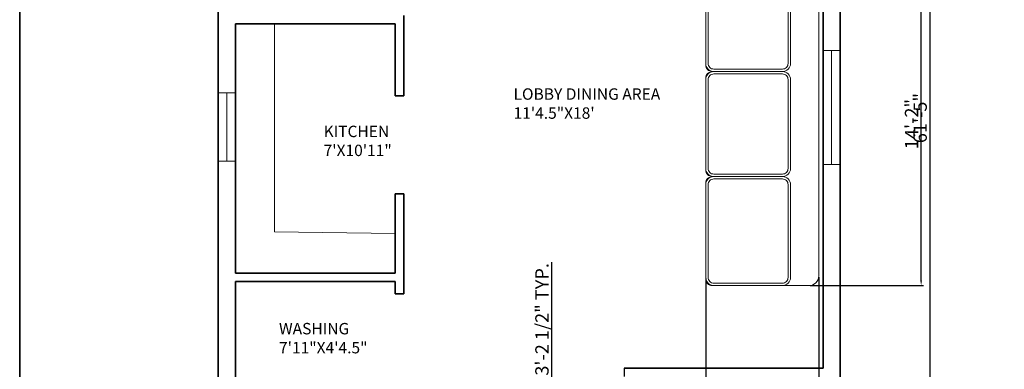
# Model space of a CAD drawing. Units: inches. Extents: x 1863 to 2938, y 1238 to 2492.
# Tile 7 of 12: x 1863 to 2381, y 1576 to 1760. Entities that reach past the tile are written whole.
import ezdxf

# ---------------------------------------------------------------- set-up
doc = ezdxf.new("R2010")
doc.units = ezdxf.units.IN
for name, color, linetype, lineweight in [('A-ANNO-DIMS', 2, 'Continuous', 18), ('A-ANNO-TTLB', 7, 'Continuous', 35), ('A-AREA-IDEN', 7, 'Continuous', 18), ('A-FLOR-FIXT', 9, 'Continuous', 18), ('A-FLOR-STRS', 7, 'Continuous', 25), ('A-FURN', 8, 'Continuous', 18), ('A-GLAZ', 4, 'Continuous', 18), ('A-WALL', 7, 'Continuous', 35)]:
    doc.layers.add(name, color=color, linetype=linetype, lineweight=lineweight)
doc.styles.get("Standard").update_dxf_attribs({"font": 'arial.ttf'})
doc.dimstyles.new('ISO-25', dxfattribs={"dimtxt": 7, "dimasz": 2.5, "dimexe": 1.25, "dimexo": 0.625, "dimtad": 1, "dimdec": 0, "dimlunit": 3, "dimtxsty": 'Standard', "dimcen": 2.5, "dimadec": 0, "dimazin": 0, "dimtfac": 1, "dimtdec": 0, "dimtmove": 0, "dimatfit": 3, "dimfxl": 1, "dimarcsym": 0})

# ---------------------------------------------------------------- blocks, each defined once
blk = doc.blocks.new('*D3')
at = {"layer": 'A-ANNO-DIMS', "color": 0, "lineweight": -2, "transparency": 16777216}
for p, q in [((2295.26, 2076.56), (2343.03, 2076.56)), ((2341.78, 2074.06), (2341.78, 1342.06)), ((2295.26, 1339.56), (2343.03, 1339.56))]:
    blk.add_line(p, q, dxfattribs=at)
at = {"layer": 'A-ANNO-DIMS', "color": 0, "transparency": 16777216}
for points in [[(2341.36, 2074.06), (2342.2, 2074.06), (2341.78, 2076.56)], [(2341.36, 1342.06), (2342.2, 1342.06), (2341.78, 1339.56)]]:
    blk.add_solid(points, dxfattribs=at)
at = {"layer": 'Defpoints', "color": 0, "transparency": 16777216}
for p in [(2294.64, 2076.56), (2294.64, 1339.56), (2341.78, 1339.56)]:
    blk.add_point(p, dxfattribs=at)
at = {"layer": 'A-ANNO-DIMS', "color": 0, "transparency": 16777216, "insert": (2337.58, 1708.06), "char_height": 7, "attachment_point": 5, "rotation": 90}
blk.add_mtext('61\'-5"', dxfattribs=at)
blk = doc.blocks.new('WIN-60')
for p, q in [((0, 60), (9, 60)), ((9, 60), (4.5, 60)), ((4.5, 60), (4.5, 0)), ((4.5, 0), (0, 0)), ((0, 0), (9, 0))]:
    blk.add_line(p, q)
blk = doc.blocks.new('WIN-36')
for p, q in [((0, 36), (9, 36)), ((9, 36), (4.5, 36)), ((4.5, 36), (4.5, 0)), ((4.5, 0), (0, 0)), ((0, 0), (9, 0))]:
    blk.add_line(p, q)
blk = doc.blocks.new('*D57')
at = {"layer": 'A-ANNO-DIMS', "color": 0, "lineweight": -2, "transparency": 16777216}
for p, q in [((2142.97, 1569.56), (2142.97, 1632.29)), ((2137.43, 1569.56), (2144.22, 1569.56)), ((2142.97, 1533.53), (2142.97, 1567.06)), ((2137.43, 1531.03), (2144.22, 1531.03))]:
    blk.add_line(p, q, dxfattribs=at)
at = {"layer": 'A-ANNO-DIMS', "color": 0, "transparency": 16777216}
for points in [[(2142.55, 1567.06), (2143.38, 1567.06), (2142.97, 1569.56)], [(2142.55, 1533.53), (2143.38, 1533.53), (2142.97, 1531.03)]]:
    blk.add_solid(points, dxfattribs=at)
at = {"layer": 'Defpoints', "color": 0, "transparency": 16777216}
for p in [(2136.81, 1569.56), (2142.97, 1569.56), (2136.81, 1531.03)]:
    blk.add_point(p, dxfattribs=at)
at = {"layer": 'A-ANNO-DIMS', "color": 0, "transparency": 16777216, "insert": (2138.72, 1602.17), "char_height": 7, "attachment_point": 5, "rotation": 90}
blk.add_mtext('3\'-2 1/2" TYP.', dxfattribs=at)
blk = doc.blocks.new('*D58')
at = {"layer": 'A-ANNO-DIMS', "color": 0, "lineweight": -2, "transparency": 16777216}
for p, q in [((2223.92, 1623.6), (2223.92, 1243.07)), ((2283.38, 1624.45), (2283.38, 1243.07)), ((2226.42, 1244.32), (2280.88, 1244.32))]:
    blk.add_line(p, q, dxfattribs=at)
at = {"layer": 'A-ANNO-DIMS', "color": 0, "transparency": 16777216}
for points in [[(2226.42, 1244.74), (2226.42, 1243.91), (2223.92, 1244.32)], [(2280.88, 1244.74), (2280.88, 1243.91), (2283.38, 1244.32)]]:
    blk.add_solid(points, dxfattribs=at)
at = {"layer": 'Defpoints', "color": 0, "transparency": 16777216}
for p in [(2223.92, 1624.22), (2283.38, 1625.07), (2283.38, 1244.32)]:
    blk.add_point(p, dxfattribs=at)
at = {"layer": 'A-ANNO-DIMS', "color": 0, "transparency": 16777216, "insert": (2253.65, 1248.57), "char_height": 7, "attachment_point": 5}
blk.add_mtext('4\'-11 1/2"', dxfattribs=at)
blk = doc.blocks.new('*D59')
at = {"layer": 'A-ANNO-DIMS', "color": 0, "lineweight": -2, "transparency": 16777216}
for p, q in [((2278.91, 1789.89), (2338.44, 1789.89)), ((2337.19, 1622.48), (2337.19, 1787.39)), ((2278.91, 1619.98), (2338.44, 1619.98))]:
    blk.add_line(p, q, dxfattribs=at)
at = {"layer": 'A-ANNO-DIMS', "color": 0, "transparency": 16777216}
for points in [[(2336.77, 1787.39), (2337.61, 1787.39), (2337.19, 1789.89)], [(2336.77, 1622.48), (2337.61, 1622.48), (2337.19, 1619.98)]]:
    blk.add_solid(points, dxfattribs=at)
at = {"layer": 'Defpoints', "color": 0, "transparency": 16777216}
for p in [(2278.29, 1789.89), (2337.19, 1789.89), (2278.29, 1619.98)]:
    blk.add_point(p, dxfattribs=at)
at = {"layer": 'A-ANNO-DIMS', "color": 0, "transparency": 16777216, "insert": (2333.05, 1704.93), "char_height": 7, "attachment_point": 5, "rotation": 90}
blk.add_mtext('14\'-2"', dxfattribs=at)

msp = doc.modelspace()

# ---------------------------------------------------------------- linework, layer by layer
at = {"layer": 'A-ANNO-TTLB'}
msp.add_lwpolyline([(1863.2, 2492.19), (2938.41, 2492.19), (2938.41, 1253.47), (1863.2, 1253.47)], close=True, dxfattribs=at)
at = {"layer": 'A-FLOR-FIXT'}
for p, q in [((1997.25, 1757.56), (1997.25, 1648.25)), ((1997.25, 1648.25), (2060.64, 1647.42))]:
    msp.add_line(p, q, dxfattribs=at)
at = {"layer": 'A-FLOR-STRS'}
msp.add_line((2181.02, 1576.56), (2181.02, 1572.06), dxfattribs=at)
at = {"layer": 'A-FURN'}
for points in [[(2228.16, 1732.54), (2264.27, 1732.54, 0.414214), (2268.52, 1736.79), (2268.52, 1785.64, 0.414214), (2264.27, 1789.89), (2228.16, 1789.89, 0.414214), (2223.92, 1785.64), (2223.92, 1736.79, 0.414214)], [(2228.16, 1733.82), (2264.27, 1733.82, 0.414214), (2267.24, 1736.79), (2267.24, 1785.64, 0.414214), (2264.27, 1788.61), (2228.16, 1788.61, 0.414214), (2225.19, 1785.64), (2225.19, 1736.79, 0.414214)], [(2228.16, 1732.54), (2264.27, 1732.54, -0.414214), (2268.52, 1728.29), (2268.52, 1681.57, -0.414214), (2264.27, 1677.32), (2228.16, 1677.32, -0.414214), (2223.92, 1681.57), (2223.92, 1728.29, -0.414214)], [(2228.16, 1731.27), (2264.27, 1731.27, -0.414214), (2267.24, 1728.29), (2267.24, 1681.57, -0.414214), (2264.27, 1678.59), (2228.16, 1678.59, -0.414214), (2225.19, 1681.57), (2225.19, 1728.29, -0.414214)], [(2228.16, 1619.98), (2264.27, 1619.98, 0.414214), (2268.52, 1624.22), (2268.52, 1673.07, 0.414214), (2264.27, 1677.32), (2228.16, 1677.32, 0.414214), (2223.92, 1673.07), (2223.92, 1624.22, 0.414214)], [(2228.16, 1621.25), (2264.27, 1621.25, 0.414214), (2267.24, 1624.22), (2267.24, 1673.07, 0.414214), (2264.27, 1676.05), (2228.16, 1676.05, 0.414214), (2225.19, 1673.07), (2225.19, 1624.22, 0.414214)]]:
    msp.add_lwpolyline(points, format="xyb", close=True, dxfattribs=at)
at = {"layer": 'A-FURN', "ltscale": 0.03}
msp.add_lwpolyline([(2223.92, 1673.88), (2223.92, 1623.37, 0.414214), (2227.31, 1619.98), (2278.29, 1619.98, 0.414214), (2283.38, 1625.07), (2283.38, 1784.79, 0.414214), (2278.29, 1789.89), (2227.31, 1789.89, 0.414214), (2223.92, 1786.49), (2223.92, 1735.98, 0.414214), (2227.31, 1732.58, -1), (2227.31, 1732.5, 0.414214), (2223.92, 1729.1), (2223.92, 1680.76, 0.414214), (2227.31, 1677.36, -1), (2227.31, 1677.28, 0.414214)], format="xyb", close=True, dxfattribs=at)
at = {"layer": 'A-WALL'}
for p, q in [((1967.64, 2076.56), (1967.64, 1339.56)), ((1967.64, 2076.56), (1967.64, 1339.56)), ((2294.64, 2076.56), (2294.64, 1495.56)), ((2285.64, 1792.56), (2285.64, 1576.56)), ((2065.14, 1762.06), (2065.14, 1757.56)), ((1976.64, 1757.56), (2060.64, 1757.56)), ((1976.64, 1757.56), (1976.64, 1626.56)), ((2060.64, 1757.56), (2060.64, 1719.81)), ((2065.14, 1757.56), (2065.14, 1719.81)), ((2060.64, 1719.81), (2065.14, 1719.81)), ((2060.64, 1668.29), (2065.14, 1668.29)), ((2060.64, 1668.29), (2060.64, 1626.56)), ((2065.14, 1668.29), (2065.14, 1615.7)), ((1976.64, 1626.56), (2060.64, 1626.56)), ((1976.64, 1622.06), (2060.64, 1622.06)), ((1976.64, 1622.06), (1976.64, 1406.06)), ((2060.64, 1622.06), (2060.64, 1615.7)), ((2060.64, 1615.7), (2065.14, 1615.7)), ((2181.02, 1576.56), (2285.64, 1576.56))]:
    msp.add_line(p, q, dxfattribs=at)

# ---------------------------------------------------------------- block references
at = {"layer": 'A-GLAZ'}
for name, p in [('WIN-60', (2285.64, 1683.62)), ('WIN-36', (1967.64, 1685.32))]:
    msp.add_blockref(name, p, dxfattribs=at)

# ---------------------------------------------------------------- texts
at = {"layer": 'A-AREA-IDEN', "char_height": 6, "attachment_point": 1}
for s, width, insert in [('LOBBY DINING AREA\\P11\'4.5"X18\'', 229.1011, (2122.87, 1723.7)), ('KITCHEN\\P7\'X10\'11"', 116.6202, (2023, 1704.05)), ('WASHING \\P7\'11"X4\'4.5"', 127.3763, (1999.54, 1600.3))]:
    msp.add_mtext_dynamic_manual_height_columns(s, width=width, gutter_width=12.5, heights=[0], dxfattribs=dict(at, insert=insert))

# ---------------------------------------------------------------- dimensions: what is measured, and where the dimension line sits
at = {"layer": 'A-ANNO-DIMS'}
for base, p1, p2, override, picture, middle in [((2341.78, 1339.56), (2294.64, 2076.56), (2294.64, 1339.56), {"dimclrd": 0, "dimclre": 0, "dimclrt": 0}, '*D3', (2337.58, 1708.06)), ((2337.19, 1789.89), (2278.29, 1619.98), (2278.29, 1789.89), {"dimdec": 1, "dimlfac": 1, "dimrnd": 0, "dimzin": 1, "dimdsep": 46, "dimlunit": 4, "dimfrac": 2}, '*D59', (2333.05, 1704.93))]:
    dim = msp.add_linear_dim(base=base, p1=p1, p2=p2, angle=90, dimstyle='ISO-25', override=override, dxfattribs=at)
    dim.commit()
    dim.dimension.update_dxf_attribs({"geometry": picture, "text_midpoint": middle})
dim = msp.add_linear_dim(base=(2142.97, 1569.56), p1=(2136.81, 1531.03), p2=(2136.81, 1569.56), angle=90, text='<> TYP.', dimstyle='ISO-25', override={"dimdec": 1, "dimlfac": 1, "dimrnd": 0, "dimzin": 1, "dimdsep": 46, "dimlunit": 4, "dimfrac": 2}, dxfattribs=at)
dim.commit()
dim.dimension.update_dxf_attribs({"geometry": '*D57', "text_midpoint": (2138.72, 1602.17)})
dim = msp.add_linear_dim(base=(2283.38, 1244.32), p1=(2223.92, 1624.22), p2=(2283.38, 1625.07), dimstyle='ISO-25', override={"dimdec": 1, "dimlfac": 1, "dimrnd": 0, "dimzin": 1, "dimdsep": 46, "dimlunit": 4, "dimfrac": 2}, dxfattribs=at)
dim.commit()
dim.dimension.update_dxf_attribs({"geometry": '*D58', "text_midpoint": (2253.65, 1248.57)})

doc.saveas('drawing.dxf')
